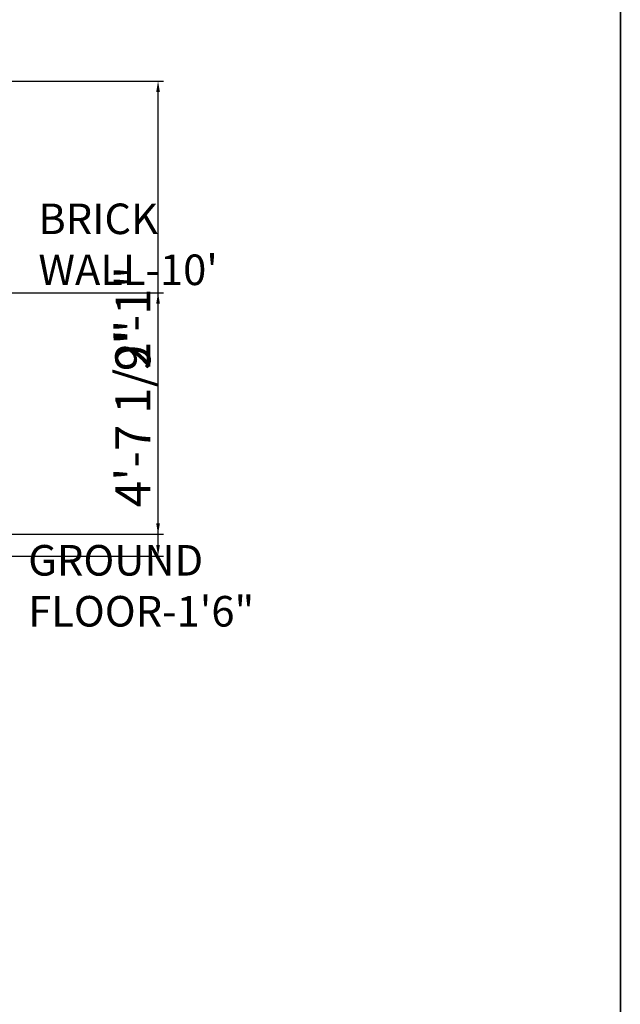
# Model space of a CAD drawing. Units: inches. Extents: x 2257 to 3678, y 834 to 1975.
# Tile 15 of 16: x 3540 to 3678, y 1594 to 1820. Entities that reach past the tile are written whole.
import ezdxf

# ---------------------------------------------------------------- set-up
doc = ezdxf.new("R2010")
doc.units = ezdxf.units.IN
for name, color, linetype, lineweight in [('A-ANNO-DIMS', 2, 'Continuous', 18), ('A-ANNO-TEXT', 7, 'Continuous', 18), ('A-ANNO-TTLB', 7, 'Continuous', 35)]:
    doc.layers.add(name, color=color, linetype=linetype, lineweight=lineweight)
doc.styles.get("Standard").update_dxf_attribs({"font": 'arial.ttf'})
doc.dimstyles.new('ISO-25', dxfattribs={"dimtxt": 8, "dimasz": 2.5, "dimexe": 1.25, "dimexo": 0.625, "dimtad": 1, "dimdec": 0, "dimlunit": 3, "dimtxsty": 'Standard', "dimcen": 2.5, "dimadec": 0, "dimazin": 0, "dimtfac": 1, "dimtdec": 0, "dimtmove": 0, "dimatfit": 3, "dimfxl": 1, "dimarcsym": 0})

# ---------------------------------------------------------------- blocks, each defined once
blk = doc.blocks.new('*D139')
at = {"layer": 'A-ANNO-DIMS', "color": 0, "lineweight": -2, "transparency": 16777216}
for p, q in [((3463.29, 1805.46), (3573.28, 1805.46)), ((3572.03, 1699.2), (3572.03, 1802.96)), ((3463.29, 1696.7), (3573.28, 1696.7))]:
    blk.add_line(p, q, dxfattribs=at)
at = {"layer": 'A-ANNO-DIMS', "color": 0, "transparency": 16777216}
for points in [[(3571.61, 1802.96), (3572.45, 1802.96), (3572.03, 1805.46)], [(3571.61, 1699.2), (3572.45, 1699.2), (3572.03, 1696.7)]]:
    blk.add_solid(points, dxfattribs=at)
at = {"layer": 'Defpoints', "color": 0, "transparency": 16777216}
for p in [(3462.66, 1805.46), (3572.03, 1805.46), (3462.66, 1696.7)]:
    blk.add_point(p, dxfattribs=at)
at = {"layer": 'A-ANNO-DIMS', "color": 0, "transparency": 16777216, "insert": (3567.32, 1751.08), "char_height": 8, "attachment_point": 5, "rotation": 90}
blk.add_mtext('9\'-1"', dxfattribs=at)
blk = doc.blocks.new('*D147')
at = {"layer": 'A-ANNO-DIMS', "color": 0, "lineweight": -2, "transparency": 16777216}
for p, q in [((3460.57, 1756.97), (3573.28, 1756.97)), ((3572.03, 1704.19), (3572.03, 1754.47)), ((3460.57, 1701.69), (3573.28, 1701.69))]:
    blk.add_line(p, q, dxfattribs=at)
at = {"layer": 'A-ANNO-DIMS', "color": 0, "transparency": 16777216}
for points in [[(3571.61, 1754.47), (3572.45, 1754.47), (3572.03, 1756.97)], [(3571.61, 1704.19), (3572.45, 1704.19), (3572.03, 1701.69)]]:
    blk.add_solid(points, dxfattribs=at)
at = {"layer": 'Defpoints', "color": 0, "transparency": 16777216}
for p in [(3459.94, 1756.97), (3572.03, 1756.97), (3459.94, 1701.69)]:
    blk.add_point(p, dxfattribs=at)
at = {"layer": 'A-ANNO-DIMS', "color": 0, "transparency": 16777216, "insert": (3567.27, 1729.33), "char_height": 8, "attachment_point": 5, "rotation": 90}
blk.add_mtext('4\'-7 1/2"', dxfattribs=at)

msp = doc.modelspace()

# ---------------------------------------------------------------- linework, layer by layer
at = {"layer": 'A-ANNO-TTLB'}
msp.add_lwpolyline([(2257.38, 1974.9), (3677.96, 1974.9), (3677.96, 849.42), (2257.38, 849.42)], close=True, dxfattribs=at)

# ---------------------------------------------------------------- texts
at = {"layer": 'A-ANNO-TEXT', "char_height": 7, "attachment_point": 1}
for s, width, insert in [("BRICK WALL-10'", 61.329, (3544.61, 1777.41)), ('GROUND FLOOR-1\'6"', 85.651, (3542.28, 1699.22))]:
    msp.add_mtext_dynamic_manual_height_columns(s, width=width, gutter_width=12.5, heights=[0], dxfattribs=dict(at, insert=insert))

# ---------------------------------------------------------------- dimensions: what is measured, and where the dimension line sits
at = {"layer": 'A-ANNO-DIMS'}
for base, p1, p2, picture, middle in [((3572.03, 1805.46), (3462.66, 1696.7), (3462.66, 1805.46), '*D139', (3567.32, 1751.08)), ((3572.03, 1756.97), (3459.94, 1701.69), (3459.94, 1756.97), '*D147', (3567.27, 1729.33))]:
    dim = msp.add_linear_dim(base=base, p1=p1, p2=p2, angle=90, dimstyle='ISO-25', override={"dimdec": 1, "dimlfac": 1, "dimrnd": 0, "dimzin": 1, "dimdsep": 46, "dimlunit": 4, "dimfrac": 2}, dxfattribs=at)
    dim.commit()
    dim.dimension.update_dxf_attribs({"geometry": picture, "text_midpoint": middle})

doc.saveas('drawing.dxf')
